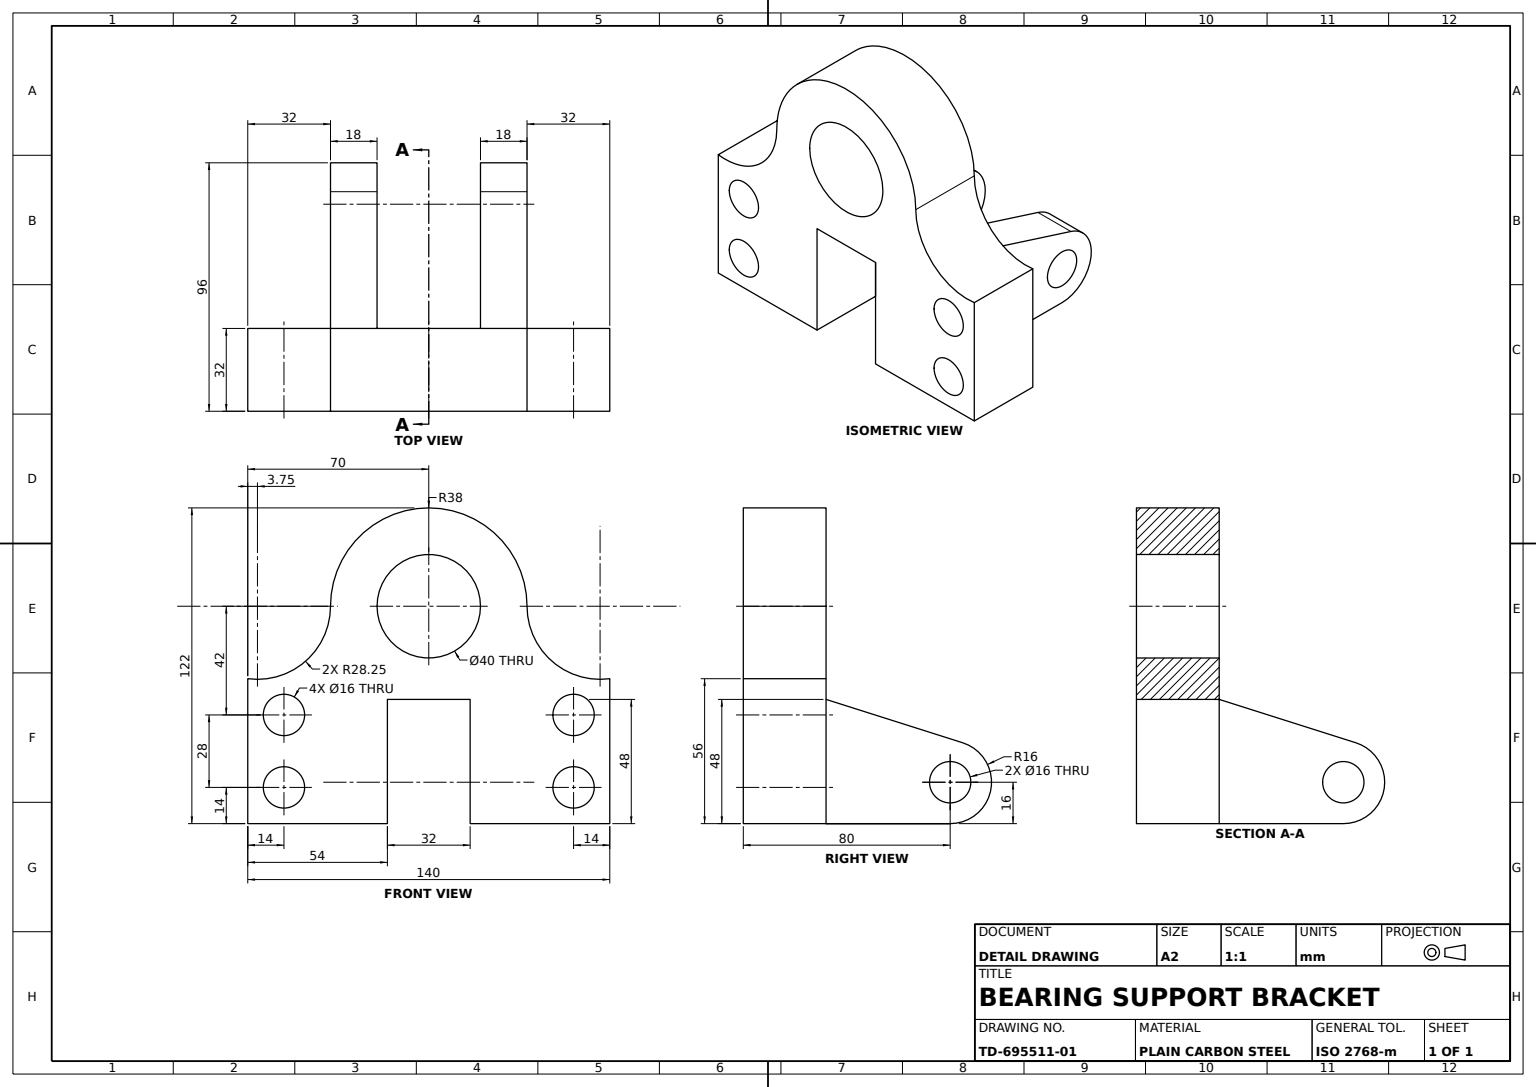
SolidWorks part; units mm, degrees
material "Plain Carbon Steel"
ref_plane "Front Plane" through (0, 0, 0) normal (0, 0, 1) x (1, 0, 0)
ref_plane "Top Plane" through (0, 0, 0) normal (0, 1, 0) x (1, 0, 0)
ref_plane "Right Plane" through (0, 0, 0) normal (1, 0, 0) x (0, 0, -1)
sketch "Bracket Body Profile" plane through (0, 0, 0) normal (0, 0, 1) x (1, 0, 0)
  line L0 (68.2963, 0) -> (-77.037, 0) construction
  line L1 (0, -61.922) -> (0, 154.2095) construction
  line L2 (-16, 0) -> (16, 0)
  line L3 (16, 0) -> (16, -48)
  line L4 (16, -48) -> (70, -48)
  line L5 (70, -48) -> (70, 8)
  line L6 (-16, -48) -> (-70, -48)
  line L7 (-70, -48) -> (-70, 8)
  line L8 (-16, 0) -> (-16, -48)
  line L9 (0, 74) -> (70, 74) construction
  arc A0 (38, 36) -> (-38, 36) centre (0, 36) ccw
  circle A1 centre (0, 36) radius 20
  arc A2 (38, 36) -> (70, 8) centre (66.25, 36) ccw
  arc A3 (-38, 36) -> (-70, 8) centre (-66.25, 36) cw
  circle A4 centre (56, -34) radius 8
  circle A5 centre (56, -6) radius 8
  circle A6 centre (-56, -34) radius 8
  circle A7 centre (-56, -6) radius 8
  point P13 (0, 0)
  dimension "D6" = 76
  dimension "D7" = 40
  dimension "D8" = 28.25
  dimension "D11" = 16
  dimension "D12" = 16
  dimension "D1" = 32
  dimension "D2" = 56
  dimension "D3" = 48
  dimension "D4" = 140
  dimension "D5" = 74
  dimension "D9" = 14
  dimension "D10" = 28
  dimension "D13" = 14
  dimension "D14" = 14
extrude "Bracket Body 32mm" add sketch "Bracket Body Profile" along normal mid plane 32
ref_plane "Lug Sketch Plane" through (20, 0, 0) normal (1, 0, 0) x (0, 0, -1)
sketch "Clevis Lug Profile" plane through (20, 0, 0) normal (1, 0, 0) x (0, 0, -1)
  line L0 (16, -48) -> (64, -48)
  line L1 (16, 0) -> (68.8347, -16.7479)
  line L2 (16, -48) -> (16, 8) construction
  line L4 (-16, -48) -> (-16, 8) construction
  line L5 (16, 0) -> (16, -48)
  arc A0 (64, -48) -> (68.8347, -16.7479) centre (64, -32) ccw
  circle A1 centre (64, -32) radius 8
  dimension "D1" = 16
  dimension "D2" = 16
  dimension "D3" = 48
  dimension "D4" = 80
extrude "Clevis Lug 18mm" add sketch "Clevis Lug Profile" along normal blind 18
mirror "Clevis Lug Mirror" about plane through (0, 0, 0) normal (1, 0, 0) of "Clevis Lug 18mm"
